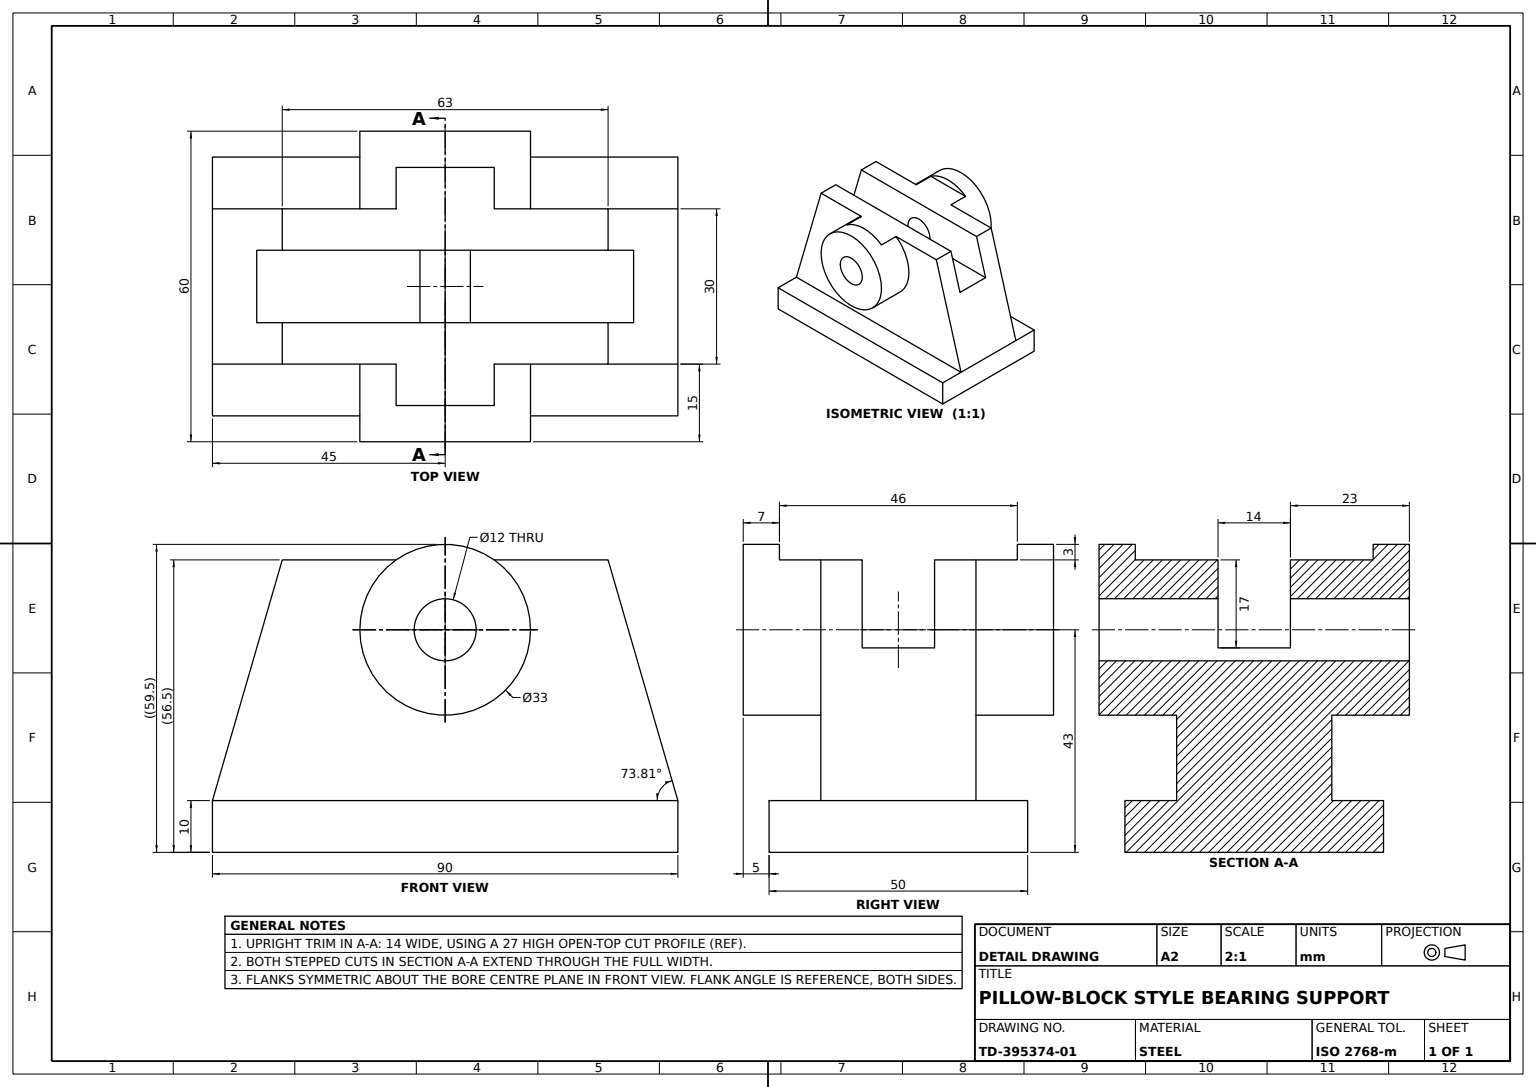
from build123d import *

# Parameters (mm, degrees)
BASE_PLATE_SKETCH_W        = 50
BASE_PLATE_SKETCH_H        = 90
BASE_PLATE_90X50X10_DEPTH  = 10
UPRIGHT_PROFILE_SKETCH_W   = 30
UPRIGHT_PROFILE_SKETCH_H   = 90
TAPERED_UPRIGHT_DEPTH      = 56.5
UPRIGHT_TRIM_SKETCH_W      = 14
UPRIGHT_TRIM_SKETCH_H      = 27
UPRIGHT_TRIM_CUT_DEPTH     = 115.661458215
BEARING_BOSS_SKETCH_R      = 16.5
BEARING_BOSS_SKETCH_R_2    = 6
BEARING_BOSS_DEPTH         = 30
CENTRE_SLOT_SKETCH_W       = 46
CENTRE_SLOT_SKETCH_H       = 10
CENTRE_SLOT_CUT_DEPTH      = 65
TOP_SLOT_CUT_DEPTH         = 65
BEARING_BORE_SKETCH_R      = 6
BEARING_BORE_THROUGH_DEPTH = 65
BOSS_NOTCH_SKETCH_W        = 14
BOSS_NOTCH_SKETCH_H        = 17
BOSS_NOTCH_CUT_DEPTH       = 65


with BuildPart() as part:
    # Base Plate Sketch → Base Plate 90x50x10 (new body)
    with BuildSketch(Plane(origin=(0, 0, 0), x_dir=(1, 0, 0), z_dir=(0, 1, 0))):
        Rectangle(BASE_PLATE_SKETCH_W, BASE_PLATE_SKETCH_H)
    extrude(amount=BASE_PLATE_90X50X10_DEPTH)

    # Upright Profile Sketch → Tapered Upright (add)
    with BuildSketch(Plane(origin=(0, 10, 0), x_dir=(1, 0, 0), z_dir=(0, 1, 0))):
        Rectangle(UPRIGHT_PROFILE_SKETCH_W, UPRIGHT_PROFILE_SKETCH_H)
    extrude(amount=TAPERED_UPRIGHT_DEPTH)

    # Upright Trim Sketch → Upright Trim Cut (cut, through all)
    with BuildSketch(Plane.XY.offset(45)):
        with Locations((0, 53)):
            Rectangle(UPRIGHT_TRIM_SKETCH_W, UPRIGHT_TRIM_SKETCH_H)
    extrude(amount=-UPRIGHT_TRIM_CUT_DEPTH, mode=Mode.SUBTRACT)

    # Bearing Boss Sketch → Bearing Boss (add, symmetric)
    with BuildSketch(Plane(origin=(0, 0, 0), x_dir=(0, 0, -1), z_dir=(1, 0, 0))):
        with Locations((0, 43)):
            Circle(BEARING_BOSS_SKETCH_R)
        with Locations((0, 43)):
            Circle(BEARING_BOSS_SKETCH_R_2, mode=Mode.SUBTRACT)
    extrude(amount=BEARING_BOSS_DEPTH, both=True)

    # Centre Slot Sketch → Centre Slot Cut (cut, symmetric)
    with BuildSketch(Plane.XY):
        with Locations((0, 61.5)):
            Rectangle(CENTRE_SLOT_SKETCH_W, CENTRE_SLOT_SKETCH_H)
    extrude(amount=CENTRE_SLOT_CUT_DEPTH, both=True, mode=Mode.SUBTRACT)

    # Top Slot Sketch → Top Slot Cut (cut, symmetric)
    with BuildSketch(Plane(origin=(0, 0, 0), x_dir=(0, 0, -1), z_dir=(1, 0, 0))):
        Polygon((-31.5, 56.5), (-45, 10), (-45, 56.5), align=None)
        Polygon((31.5, 56.5), (45, 10), (45, 56.5), align=None)
    extrude(amount=TOP_SLOT_CUT_DEPTH, both=True, mode=Mode.SUBTRACT)

    # Bearing Bore Sketch → Bearing Bore Through (cut, symmetric)
    with BuildSketch(Plane.ZY.offset(15)):
        with Locations(Location((0, 43, 0), (0, 0, 180))):
            Circle(BEARING_BORE_SKETCH_R)
    extrude(amount=BEARING_BORE_THROUGH_DEPTH, both=True, mode=Mode.SUBTRACT)

    # Boss Notch Sketch → Boss Notch Cut (cut, symmetric)
    with BuildSketch(Plane.XY):
        with Locations((0, 48)):
            Rectangle(BOSS_NOTCH_SKETCH_W, BOSS_NOTCH_SKETCH_H)
    extrude(amount=BOSS_NOTCH_CUT_DEPTH, both=True, mode=Mode.SUBTRACT)


solid = part.part
